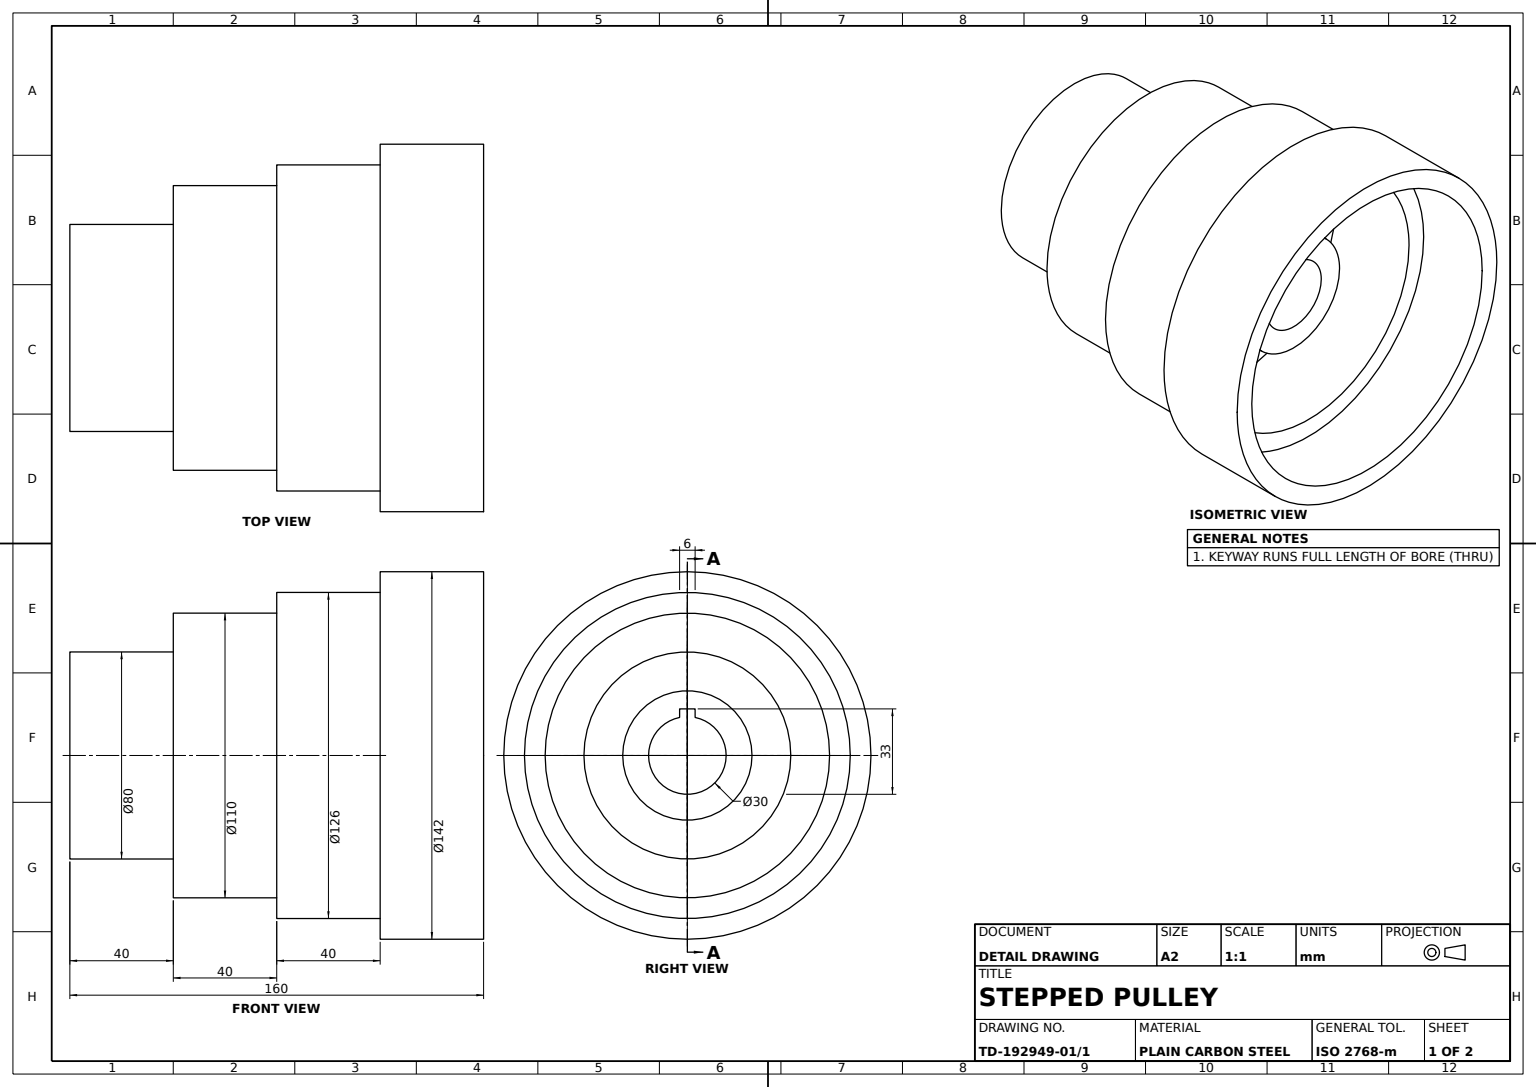
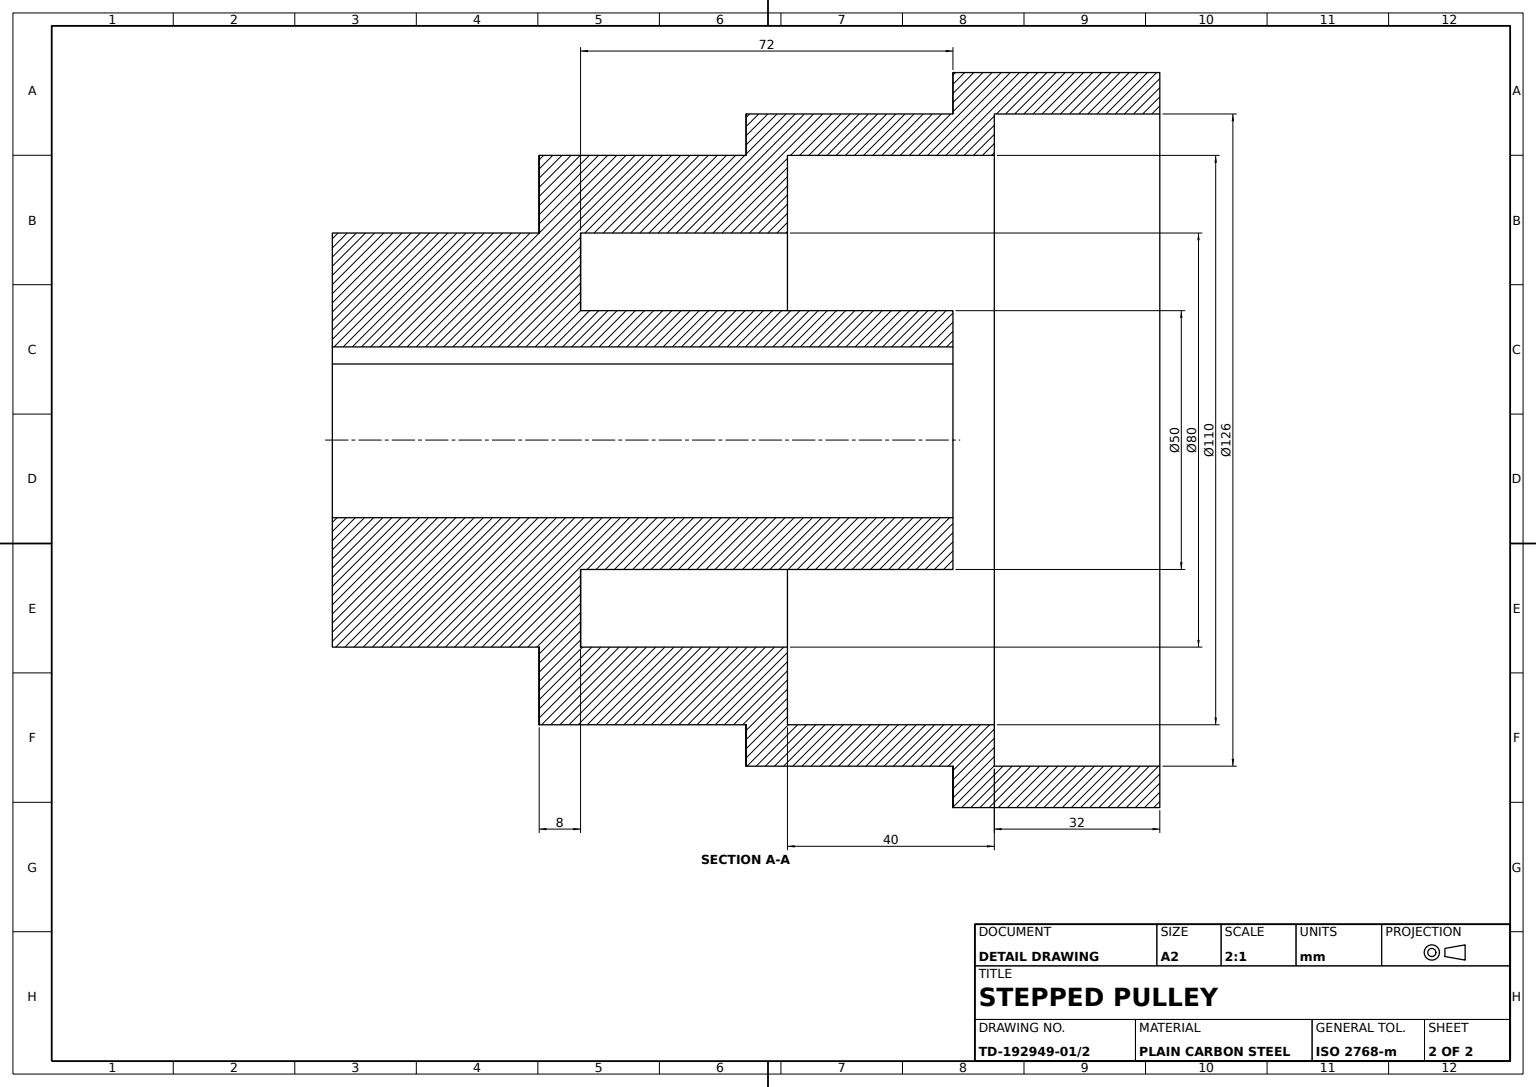
from build123d import *

# Parameters (mm, degrees)
KEYWAY_PROFILE_6X6_W = 6
KEYWAY_PROFILE_6X6_H = 6
KEYWAY_CUT_6X6_DEPTH = 211


with BuildPart() as part:
    # Pulley Step Profile → Stepped Pulley Body (revolve)
    with BuildSketch(Plane.XY, mode=Mode.PRIVATE) as stepped_pulley_body_sk:
        Polygon((0, 40), (0, 15), (120, 15), (120, 25), (48, 25), (48, 40), (88, 40), (88, 55), (128, 55), (128, 63), (160, 63), (160, 71), (120, 71), (120, 63), (80, 63), (80, 55), (40, 55), (40, 40), align=None)
    revolve(stepped_pulley_body_sk.sketch.rotate(Axis((-51.578947368, 0, 0), (1, 0, 0)), 90), axis=Axis((-51.578947368, 0, 0), (1, 0, 0)))

    # Keyway Profile 6x6 → Keyway Cut 6x6 (cut)
    with BuildSketch(Plane.ZY):
        with Locations((0, 15)):
            Rectangle(KEYWAY_PROFILE_6X6_W, KEYWAY_PROFILE_6X6_H)
    extrude(amount=-KEYWAY_CUT_6X6_DEPTH, mode=Mode.SUBTRACT)


solid = part.part
